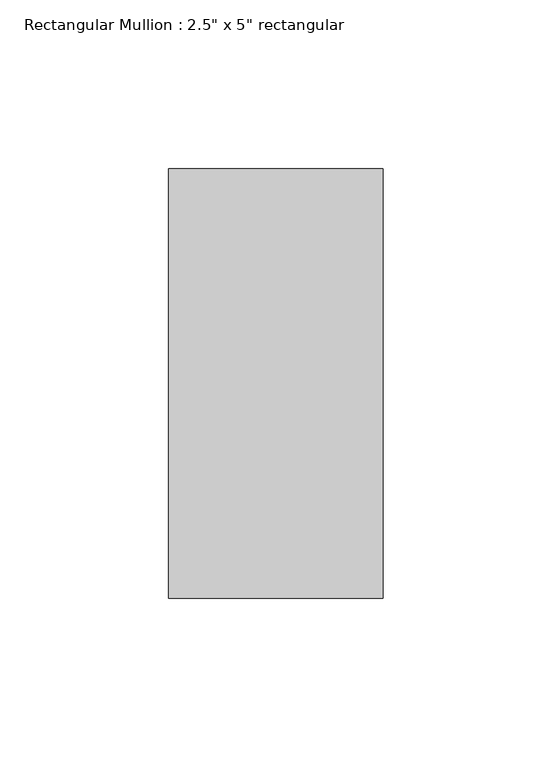
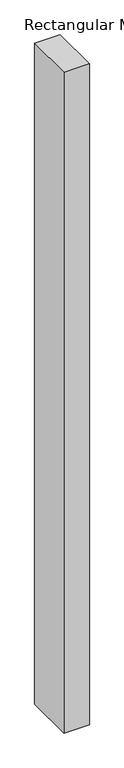
"""IFC4 building model written with IfcOpenShell, lengths in millimetres: member geometry."""

from ifc_helpers import new_model, si_unit, frame, origin, place, context, project, spatial, polyline, outline, extrude, source, transform, mapped, element, save


def member_dded4e1f(model_context):
    return source(origin(), model_context, "Body", "SweptSolid", [
        extrude(outline(polyline([(31.75, 63.5), (31.75, -63.5), (-31.75, -63.5), (-31.75, 63.5), (31.75, 63.5)])), frame((0.0, 0.0, -1750.3622634), z_axis=(0.0, 0.0, 1.0), x_axis=(1.0, 0.0, 0.0)), (0.0, 0.0, 1.0), 1750.3622634),
    ])


if __name__ == "__main__":
    model = new_model("IFC4")
    model_context = context("Model", 3, world=origin())
    ifc_project = project(units=[si_unit("LENGTHUNIT", "METRE", prefix="MILLI")], contexts=[model_context])
    site = spatial("IfcSite", under=ifc_project)
    building = spatial("IfcBuilding", under=site)
    placement = place(None, origin())
    member_shape = member_dded4e1f(model_context)
    element("IfcMember", 1, ObjectType="Rectangular Mullion : 2.5\" x 5\" rectangular", at=placement, inside=building, context=model_context, shape_type="MappedRepresentation", body=[
        mapped(member_shape, transform((0.0, 0.0, 0.0), x_axis=(1.0, 0.0, 0.0), y_axis=(0.0, 1.0, 0.0), z_axis=(0.0, 0.0, 1.0))),
    ])
    save(model, "model.ifc")

# Revit data of these elements
# Type "Rectangular Mullion : 2.5\" x 5\" rectangular"
#   built-in parameter 1007304 = 0.416667 (stored number, unit not read)
#   built-in parameter 1007301 = 0.104167 (stored number, unit not read)
#   built-in parameter 1007300 = 0.104167 (stored number, unit not read)
# Element 1 (IfcMember, "Rectangular Mullion : 2.5\" x 5\" rectangular")
#   Materials on its faces: "Aluminum"
# Materials
#   "Aluminum": class "Metal", colour RGB 247 247 247, transparency 0, Description = "Aluminum 6061", Cost = 0
